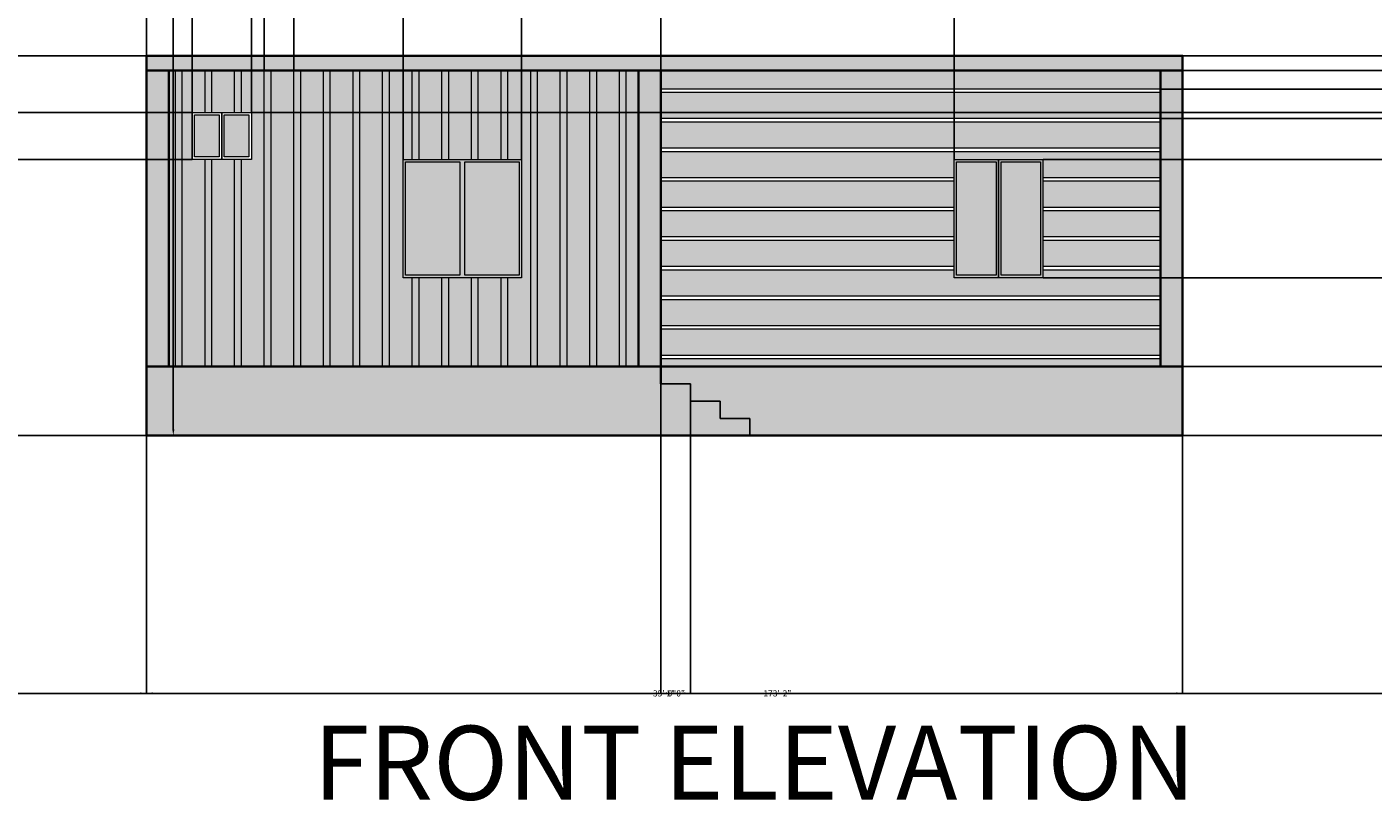
# Model space of a CAD drawing. Units: inches. Extents: x 481 to 2783, y 1975 to 3327.
# Tile 4 of 13: x 1326 to 1872, y 1975 to 2289. Entities that reach past the tile are written whole.
import ezdxf

# ---------------------------------------------------------------- set-up
doc = ezdxf.new("R2010")
doc.units = ezdxf.units.IN
doc.header["$MEASUREMENT"] = 0
for name, color, linetype, lineweight in [('A-ANNO-DIMS', 50, 'Continuous', 18), ('A-ANNO-TEXT', 50, 'Continuous', 30), ('A-ELEV', 7, 'Continuous', 35), ('A-ELEV-CLAD', 7, 'Continuous', 13), ('A-ELEV-CONC-PATT', 8, 'Continuous', 13), ('A-ELEV-FRAM-PATT', 8, 'Continuous', 13), ('A-ELEV-GLAZ', 7, 'Continuous', 20), ('A-ELEV-GLAZ-PATT', 7, 'Continuous', 13), ('A-ELEV-STRS', 7, 'Continuous', 25), ('C-TOPO', 7, 'Continuous', 25)]:
    doc.layers.add(name, color=color, linetype=linetype, lineweight=lineweight)
for name, color, linetype, lineweight, true_color in [('A-ELEV-CLAD-PATT', 141, 'Continuous', 13, 0xadddf7), ('A-ELEV-PIER-PATT', 251, 'Continuous', 13, 0x636466), ('A-ELEV-WALL-PATT', 143, 'Continuous', 13, 0x7aafdf)]:
    doc.layers.add(name, color=color, linetype=linetype, lineweight=lineweight, true_color=true_color)
doc.styles.get("Standard").update_dxf_attribs({"font": 'arial.ttf'})
doc.dimstyles.get("Standard").update_dxf_attribs({"dimtxt": 2.5, "dimasz": 2.5, "dimexe": 0.18, "dimexo": 0.0625, "dimgap": 0.09, "dimtad": 0, "dimtih": 1, "dimtoh": 1, "dimzin": 0, "dimdsep": 46, "dimlunit": 3, "dimtxsty": 'Standard', "dimcen": 0.09, "dimadec": 0, "dimazin": 0, "dimtfac": 1, "dimtofl": 0, "dimtmove": 0, "dimatfit": 3, "dimfxl": 1, "dimtolj": 1, "dimtzin": 0, "dimarcsym": 0})
pattern_1 = [(50, (0, 162.5314), (7.172602, -0.627521), [0.75, -8.25]), (355, (0, 162.531), (-1.387513, 7.521921), [0.6, -6.6]), (100.45144, (0.598, 162.479), (5.785088, 6.8944), [0.637402, -7.011421]), (46.1842, (0, 164.531), (10.672413, -1.655193), [1.125, -12.375]), (96.63564, (0.889, 164.393), (9.34662, 9.741186), [0.956103, -10.517138]), (351.18416, (0, 164.531), (9.34662, 9.741186), [0.9, -9.9]), (21, (1, 164.0314), (5.96907, -4.026189), [0.75, -8.25]), (326, (1, 164.031), (2.433153, 7.2515), [0.6, -6.6]), (71.45144, (1.4974, 163.696), (8.402224, 3.225312), [0.637402, -7.011421]), (37.5, (0, 162.5314), (0.1215986, 3.3289385), [0, -6.52, 0, -6.7, 0, -6.625]), (7.5, (0, 162.5314), (2.6306954, 3.944117), [0, -3.82, 0, -6.37, 0, -2.525]), (327.5, (-2.23, 162.5314), (5.3382244, -0.2255487), [0, -2.5, 0, -7.8, 0, -10.35]), (317.5, (-3.23, 162.5314), (5.831862, 1.00105), [0, -3.25, 0, -5.18, 0, -7.35])]

# ---------------------------------------------------------------- blocks, each defined once
blk = doc.blocks.new('*D54')
at = {"layer": 'A-ANNO-DIMS', "color": 0, "lineweight": -2, "transparency": 16777216}
for p, q in [((1324.1, 2531.22), (1385.48, 2531.22)), ((1385.3, 2528.72), (1385.3, 2328.4)), ((1385.3, 2125.32), (1385.3, 2325.64)), ((1324.1, 2122.82), (1385.48, 2122.82))]:
    blk.add_line(p, q, dxfattribs=at)
at = {"layer": 'A-ANNO-DIMS', "color": 0, "transparency": 16777216}
for points in [[(1384.88, 2528.72), (1385.72, 2528.72), (1385.3, 2531.22)], [(1384.88, 2125.32), (1385.72, 2125.32), (1385.3, 2122.82)]]:
    blk.add_solid(points, dxfattribs=at)
at = {"layer": 'Defpoints', "color": 0, "transparency": 16777216}
for p in [(1324.04, 2531.22), (1385.3, 2531.22), (1324.04, 2122.82)]:
    blk.add_point(p, dxfattribs=at)
at = {"layer": 'A-ANNO-DIMS', "color": 0, "transparency": 16777216, "insert": (1385.3, 2327.02), "char_height": 2.5, "attachment_point": 5}
blk.add_mtext('\\A1;PALM 34\'-0 1/2"', dxfattribs=at)
blk = doc.blocks.new('*D66')
at = {"layer": 'A-ANNO-DIMS', "color": 0, "lineweight": -2, "transparency": 16777216}
for p, q in [((591.06, 2122.76), (591.06, 2018.14)), ((2669.26, 2122.76), (2669.26, 2018.14)), ((593.56, 2018.32), (1624.92, 2018.32)), ((2666.76, 2018.32), (1635.4, 2018.32))]:
    blk.add_line(p, q, dxfattribs=at)
at = {"layer": 'A-ANNO-DIMS', "color": 0, "transparency": 16777216}
for points in [[(593.56, 2018.74), (593.56, 2017.9), (591.06, 2018.32)], [(2666.76, 2018.74), (2666.76, 2017.9), (2669.26, 2018.32)]]:
    blk.add_solid(points, dxfattribs=at)
at = {"layer": 'Defpoints', "color": 0, "transparency": 16777216}
for p in [(591.06, 2122.82), (2669.26, 2122.82), (2669.26, 2018.32)]:
    blk.add_point(p, dxfattribs=at)
at = {"layer": 'A-ANNO-DIMS', "color": 0, "transparency": 16777216, "insert": (1630.16, 2018.32), "char_height": 2.5, "attachment_point": 5}
blk.add_mtext('\\A1;173\'-2"', dxfattribs=at)
blk = doc.blocks.new('*D67')
at = {"layer": 'A-ANNO-DIMS', "color": 0, "lineweight": -2, "transparency": 16777216}
for p, q in [((591.06, 2122.76), (591.06, 2018.14)), ((1374.44, 2122.76), (1374.44, 2018.14)), ((593.56, 2018.32), (975.45, 2018.32)), ((1371.94, 2018.32), (990.05, 2018.32))]:
    blk.add_line(p, q, dxfattribs=at)
at = {"layer": 'A-ANNO-DIMS', "color": 0, "transparency": 16777216}
for points in [[(593.56, 2018.74), (593.56, 2017.9), (591.06, 2018.32)], [(1371.94, 2018.74), (1371.94, 2017.9), (1374.44, 2018.32)]]:
    blk.add_solid(points, dxfattribs=at)
at = {"layer": 'Defpoints', "color": 0, "transparency": 16777216}
for p in [(591.06, 2122.82), (1374.44, 2122.82), (1374.44, 2018.32)]:
    blk.add_point(p, dxfattribs=at)
at = {"layer": 'A-ANNO-DIMS', "color": 0, "transparency": 16777216, "insert": (982.75, 2018.32), "char_height": 2.5, "attachment_point": 5}
blk.add_mtext('\\A1;65\'-3 1/2"', dxfattribs=at)
blk = doc.blocks.new('*D68')
at = {"layer": 'A-ANNO-DIMS', "color": 0, "lineweight": -2, "transparency": 16777216}
for p, q in [((1374.44, 2122.76), (1374.44, 2018.14)), ((1794.44, 2122.76), (1794.44, 2018.14)), ((1376.94, 2018.32), (1580.05, 2018.32)), ((1791.94, 2018.32), (1588.82, 2018.32))]:
    blk.add_line(p, q, dxfattribs=at)
at = {"layer": 'A-ANNO-DIMS', "color": 0, "transparency": 16777216}
for points in [[(1376.94, 2018.74), (1376.94, 2017.9), (1374.44, 2018.32)], [(1791.94, 2018.74), (1791.94, 2017.9), (1794.44, 2018.32)]]:
    blk.add_solid(points, dxfattribs=at)
at = {"layer": 'Defpoints', "color": 0, "transparency": 16777216}
for p in [(1374.44, 2122.82), (1794.44, 2122.82), (1794.44, 2018.32)]:
    blk.add_point(p, dxfattribs=at)
at = {"layer": 'A-ANNO-DIMS', "color": 0, "transparency": 16777216, "insert": (1584.44, 2018.32), "char_height": 2.5, "attachment_point": 5}
blk.add_mtext('\\A1;35\'-0"', dxfattribs=at)
blk = doc.blocks.new('*D69')
at = {"layer": 'A-ANNO-DIMS', "color": 0, "lineweight": -2, "transparency": 16777216}
for p, q in [((1374.38, 2276.82), (486.38, 2276.82)), ((486.56, 2274.32), (486.56, 2201.19)), ((486.56, 2125.32), (486.56, 2198.45)), ((1374.38, 2122.82), (486.38, 2122.82))]:
    blk.add_line(p, q, dxfattribs=at)
at = {"layer": 'A-ANNO-DIMS', "color": 0, "transparency": 16777216}
for points in [[(486.15, 2274.32), (486.98, 2274.32), (486.56, 2276.82)], [(486.15, 2125.32), (486.98, 2125.32), (486.56, 2122.82)]]:
    blk.add_solid(points, dxfattribs=at)
at = {"layer": 'Defpoints', "color": 0, "transparency": 16777216}
for p in [(486.56, 2276.82), (1374.44, 2276.82), (1374.44, 2122.82)]:
    blk.add_point(p, dxfattribs=at)
at = {"layer": 'A-ANNO-DIMS', "color": 0, "transparency": 16777216, "insert": (486.56, 2199.82), "char_height": 2.5, "attachment_point": 5}
blk.add_mtext('\\A1;12\'-10"', dxfattribs=at)
blk = doc.blocks.new('*D70')
at = {"layer": 'A-ANNO-DIMS', "color": 0, "lineweight": -2, "transparency": 16777216}
for p, q in [((1794.5, 2150.82), (2773.94, 2150.82)), ((2773.76, 2148.32), (2773.76, 2138.17)), ((2773.76, 2125.32), (2773.76, 2135.48)), ((1794.5, 2122.82), (2773.94, 2122.82))]:
    blk.add_line(p, q, dxfattribs=at)
at = {"layer": 'A-ANNO-DIMS', "color": 0, "transparency": 16777216}
for points in [[(2773.34, 2148.32), (2774.17, 2148.32), (2773.76, 2150.82)], [(2773.34, 2125.32), (2774.17, 2125.32), (2773.76, 2122.82)]]:
    blk.add_solid(points, dxfattribs=at)
at = {"layer": 'Defpoints', "color": 0, "transparency": 16777216}
for p in [(1794.44, 2150.82), (2773.76, 2150.82), (1794.44, 2122.82)]:
    blk.add_point(p, dxfattribs=at)
at = {"layer": 'A-ANNO-DIMS', "color": 0, "transparency": 16777216, "insert": (2773.76, 2136.82), "char_height": 2.5, "attachment_point": 5}
blk.add_mtext('\\A1;2\'-4"', dxfattribs=at)
blk = doc.blocks.new('*D71')
at = {"layer": 'A-ANNO-DIMS', "color": 0, "lineweight": -2, "transparency": 16777216}
for p, q in [((1737.9, 2186.82), (2773.94, 2186.82)), ((2773.76, 2184.32), (2773.76, 2170.19)), ((2773.76, 2153.32), (2773.76, 2167.45)), ((1794.5, 2150.82), (2773.94, 2150.82))]:
    blk.add_line(p, q, dxfattribs=at)
at = {"layer": 'A-ANNO-DIMS', "color": 0, "transparency": 16777216}
for points in [[(2773.34, 2184.32), (2774.17, 2184.32), (2773.76, 2186.82)], [(2773.34, 2153.32), (2774.17, 2153.32), (2773.76, 2150.82)]]:
    blk.add_solid(points, dxfattribs=at)
at = {"layer": 'Defpoints', "color": 0, "transparency": 16777216}
for p in [(1737.84, 2186.82), (2773.76, 2186.82), (1794.44, 2150.82)]:
    blk.add_point(p, dxfattribs=at)
at = {"layer": 'A-ANNO-DIMS', "color": 0, "transparency": 16777216, "insert": (2773.76, 2168.82), "char_height": 2.5, "attachment_point": 5}
blk.add_mtext('\\A1;3\'-0"', dxfattribs=at)
blk = doc.blocks.new('*D72')
at = {"layer": 'A-ANNO-DIMS', "color": 0, "lineweight": -2, "transparency": 16777216}
for p, q in [((1737.9, 2234.82), (2773.94, 2234.82)), ((2773.76, 2232.32), (2773.76, 2212.19)), ((2773.76, 2189.32), (2773.76, 2209.45)), ((1737.9, 2186.82), (2773.94, 2186.82))]:
    blk.add_line(p, q, dxfattribs=at)
at = {"layer": 'A-ANNO-DIMS', "color": 0, "transparency": 16777216}
for points in [[(2773.34, 2232.32), (2774.17, 2232.32), (2773.76, 2234.82)], [(2773.34, 2189.32), (2774.17, 2189.32), (2773.76, 2186.82)]]:
    blk.add_solid(points, dxfattribs=at)
at = {"layer": 'Defpoints', "color": 0, "transparency": 16777216}
for p in [(1737.84, 2234.82), (2773.76, 2234.82), (1737.84, 2186.82)]:
    blk.add_point(p, dxfattribs=at)
at = {"layer": 'A-ANNO-DIMS', "color": 0, "transparency": 16777216, "insert": (2773.76, 2210.82), "char_height": 2.5, "attachment_point": 5}
blk.add_mtext('\\A1;4\'-0"', dxfattribs=at)
blk = doc.blocks.new('*D73')
at = {"layer": 'A-ANNO-DIMS', "color": 0, "lineweight": -2, "transparency": 16777216}
for p, q in [((1392.88, 2253.82), (486.38, 2253.82)), ((486.56, 2251.32), (486.56, 2245.67)), ((486.56, 2237.32), (486.56, 2242.98)), ((1392.88, 2234.82), (486.38, 2234.82))]:
    blk.add_line(p, q, dxfattribs=at)
at = {"layer": 'A-ANNO-DIMS', "color": 0, "transparency": 16777216}
for points in [[(486.15, 2251.32), (486.98, 2251.32), (486.56, 2253.82)], [(486.15, 2237.32), (486.98, 2237.32), (486.56, 2234.82)]]:
    blk.add_solid(points, dxfattribs=at)
at = {"layer": 'Defpoints', "color": 0, "transparency": 16777216}
for p in [(486.56, 2253.82), (1392.94, 2253.82), (1392.94, 2234.82)]:
    blk.add_point(p, dxfattribs=at)
at = {"layer": 'A-ANNO-DIMS', "color": 0, "transparency": 16777216, "insert": (486.56, 2244.32), "char_height": 2.5, "attachment_point": 5}
blk.add_mtext('\\A1;1\'-7"', dxfattribs=at)
blk = doc.blocks.new('*D74')
at = {"layer": 'A-ANNO-DIMS', "color": 0, "lineweight": -2, "transparency": 16777216}
for p, q in [((1412.86, 2270.82), (2773.94, 2270.82)), ((2773.76, 2268.32), (2773.76, 2263.69)), ((2773.76, 2256.32), (2773.76, 2260.95)), ((1417, 2253.82), (2773.94, 2253.82))]:
    blk.add_line(p, q, dxfattribs=at)
at = {"layer": 'A-ANNO-DIMS', "color": 0, "transparency": 16777216}
for points in [[(2773.34, 2268.32), (2774.17, 2268.32), (2773.76, 2270.82)], [(2773.34, 2256.32), (2774.17, 2256.32), (2773.76, 2253.82)]]:
    blk.add_solid(points, dxfattribs=at)
at = {"layer": 'Defpoints', "color": 0, "transparency": 16777216}
for p in [(1412.79, 2270.82), (2773.76, 2270.82), (1416.94, 2253.82)]:
    blk.add_point(p, dxfattribs=at)
at = {"layer": 'A-ANNO-DIMS', "color": 0, "transparency": 16777216, "insert": (2773.76, 2262.32), "char_height": 2.5, "attachment_point": 5}
blk.add_mtext('\\A1;1\'-5"', dxfattribs=at)
blk = doc.blocks.new('*D75')
at = {"layer": 'A-ANNO-DIMS', "color": 0, "lineweight": -2, "transparency": 16777216}
for p, q in [((1794.5, 2276.82), (2773.94, 2276.82)), ((2773.76, 2276.82), (2773.76, 2279.32)), ((2773.76, 2279.32), (2776.26, 2279.32)), ((1794.5, 2270.82), (2773.94, 2270.82)), ((2773.76, 2273.32), (2773.76, 2274.32))]:
    blk.add_line(p, q, dxfattribs=at)
at = {"layer": 'A-ANNO-DIMS', "color": 0, "transparency": 16777216}
for points in [[(2773.34, 2274.32), (2774.17, 2274.32), (2773.76, 2276.82)], [(2773.34, 2273.32), (2774.17, 2273.32), (2773.76, 2270.82)]]:
    blk.add_solid(points, dxfattribs=at)
at = {"layer": 'Defpoints', "color": 0, "transparency": 16777216}
for p in [(1794.44, 2276.82), (2773.76, 2276.82), (1794.44, 2270.82)]:
    blk.add_point(p, dxfattribs=at)
at = {"layer": 'A-ANNO-DIMS', "color": 0, "transparency": 16777216, "insert": (2779.67, 2279.32), "char_height": 2.5, "attachment_point": 5}
blk.add_mtext('\\A1;0\'-6"', dxfattribs=at)
blk = doc.blocks.new('*D76')
at = {"layer": 'A-ANNO-DIMS', "color": 0, "lineweight": -2, "transparency": 16777216}
for p, q in [((1374.44, 2276.88), (1374.44, 2651.23)), ((1376.94, 2651.05), (1377.48, 2651.05)), ((1390.44, 2651.05), (1389.9, 2651.05)), ((1392.94, 2253.88), (1392.94, 2651.23))]:
    blk.add_line(p, q, dxfattribs=at)
at = {"layer": 'A-ANNO-DIMS', "color": 0, "transparency": 16777216}
for points in [[(1376.94, 2651.47), (1376.94, 2650.64), (1374.44, 2651.05)], [(1390.44, 2651.47), (1390.44, 2650.64), (1392.94, 2651.05)]]:
    blk.add_solid(points, dxfattribs=at)
at = {"layer": 'Defpoints', "color": 0, "transparency": 16777216}
for p in [(1392.94, 2651.05), (1374.44, 2276.82), (1392.94, 2253.82)]:
    blk.add_point(p, dxfattribs=at)
at = {"layer": 'A-ANNO-DIMS', "color": 0, "transparency": 16777216, "insert": (1383.69, 2651.05), "char_height": 2.5, "attachment_point": 5}
blk.add_mtext('\\A1;1\'-6 1/2"', dxfattribs=at)
blk = doc.blocks.new('*D77')
at = {"layer": 'A-ANNO-DIMS', "color": 0, "lineweight": -2, "transparency": 16777216}
for p, q in [((1416.94, 2253.88), (1416.94, 2651.23)), ((1419.44, 2651.05), (1441.36, 2651.05)), ((1475.94, 2651.05), (1454.01, 2651.05)), ((1478.44, 2234.88), (1478.44, 2651.23))]:
    blk.add_line(p, q, dxfattribs=at)
at = {"layer": 'A-ANNO-DIMS', "color": 0, "transparency": 16777216}
for points in [[(1419.44, 2651.47), (1419.44, 2650.64), (1416.94, 2651.05)], [(1475.94, 2651.47), (1475.94, 2650.64), (1478.44, 2651.05)]]:
    blk.add_solid(points, dxfattribs=at)
at = {"layer": 'Defpoints', "color": 0, "transparency": 16777216}
for p in [(1478.44, 2651.05), (1416.94, 2253.82), (1478.44, 2234.82)]:
    blk.add_point(p, dxfattribs=at)
at = {"layer": 'A-ANNO-DIMS', "color": 0, "transparency": 16777216, "insert": (1447.69, 2651.05), "char_height": 2.5, "attachment_point": 5}
blk.add_mtext('\\A1;5\'-1 1/2"', dxfattribs=at)
blk = doc.blocks.new('*D78')
at = {"layer": 'A-ANNO-DIMS', "color": 0, "lineweight": -2, "transparency": 16777216}
for p, q in [((1526.44, 2234.88), (1526.44, 2651.23)), ((1528.94, 2651.05), (1548.31, 2651.05)), ((1580.44, 2651.05), (1561.06, 2651.05)), ((1582.94, 2270.88), (1582.94, 2651.23))]:
    blk.add_line(p, q, dxfattribs=at)
at = {"layer": 'A-ANNO-DIMS', "color": 0, "transparency": 16777216}
for points in [[(1528.94, 2651.47), (1528.94, 2650.64), (1526.44, 2651.05)], [(1580.44, 2651.47), (1580.44, 2650.64), (1582.94, 2651.05)]]:
    blk.add_solid(points, dxfattribs=at)
at = {"layer": 'Defpoints', "color": 0, "transparency": 16777216}
for p in [(1582.94, 2651.05), (1582.94, 2270.82), (1526.44, 2234.82)]:
    blk.add_point(p, dxfattribs=at)
at = {"layer": 'A-ANNO-DIMS', "color": 0, "transparency": 16777216, "insert": (1554.69, 2651.05), "char_height": 2.5, "attachment_point": 5}
blk.add_mtext('\\A1;4\'-8 1/2"', dxfattribs=at)
blk = doc.blocks.new('*D79')
at = {"layer": 'A-ANNO-DIMS', "color": 0, "lineweight": -2, "transparency": 16777216}
for p, q in [((1582.94, 2270.88), (1582.94, 2651.23)), ((1585.44, 2651.05), (1638.01, 2651.05)), ((1699.34, 2651.05), (1646.77, 2651.05)), ((1701.84, 2234.88), (1701.84, 2651.23))]:
    blk.add_line(p, q, dxfattribs=at)
at = {"layer": 'A-ANNO-DIMS', "color": 0, "transparency": 16777216}
for points in [[(1585.44, 2651.47), (1585.44, 2650.64), (1582.94, 2651.05)], [(1699.34, 2651.47), (1699.34, 2650.64), (1701.84, 2651.05)]]:
    blk.add_solid(points, dxfattribs=at)
at = {"layer": 'Defpoints', "color": 0, "transparency": 16777216}
for p in [(1701.84, 2651.05), (1582.94, 2270.82), (1701.84, 2234.82)]:
    blk.add_point(p, dxfattribs=at)
at = {"layer": 'A-ANNO-DIMS', "color": 0, "transparency": 16777216, "insert": (1642.39, 2651.05), "char_height": 2.5, "attachment_point": 5}
blk.add_mtext('\\A1;9\'-11"', dxfattribs=at)
blk = doc.blocks.new('*D80')
at = {"layer": 'A-ANNO-DIMS', "color": 0, "lineweight": -2, "transparency": 16777216}
for p, q in [((1582.94, 2150.76), (1582.94, 2018.14)), ((1594.94, 2143.76), (1594.94, 2018.14)), ((1585.44, 2018.32), (1585.64, 2018.32)), ((1592.44, 2018.32), (1592.23, 2018.32))]:
    blk.add_line(p, q, dxfattribs=at)
at = {"layer": 'A-ANNO-DIMS', "color": 0, "transparency": 16777216}
for points in [[(1585.44, 2018.74), (1585.44, 2017.9), (1582.94, 2018.32)], [(1592.44, 2018.74), (1592.44, 2017.9), (1594.94, 2018.32)]]:
    blk.add_solid(points, dxfattribs=at)
at = {"layer": 'Defpoints', "color": 0, "transparency": 16777216}
for p in [(1582.94, 2150.82), (1594.94, 2143.82), (1582.94, 2018.32)]:
    blk.add_point(p, dxfattribs=at)
at = {"layer": 'A-ANNO-DIMS', "color": 0, "transparency": 16777216, "insert": (1588.94, 2018.32), "char_height": 2.5, "attachment_point": 5}
blk.add_mtext('\\A1;1\'-0"', dxfattribs=at)
blk = doc.blocks.new('*D81')
at = {"layer": 'A-ANNO-DIMS', "color": 0, "lineweight": -2, "transparency": 16777216}
for p, q in [((1422.16, 2270.88), (1422.16, 2651.23)), ((1424.66, 2651.05), (1424.87, 2651.05)), ((1431.66, 2651.05), (1431.46, 2651.05)), ((1434.16, 2270.88), (1434.16, 2651.23))]:
    blk.add_line(p, q, dxfattribs=at)
at = {"layer": 'A-ANNO-DIMS', "color": 0, "transparency": 16777216}
for points in [[(1424.66, 2651.47), (1424.66, 2650.64), (1422.16, 2651.05)], [(1431.66, 2651.47), (1431.66, 2650.64), (1434.16, 2651.05)]]:
    blk.add_solid(points, dxfattribs=at)
at = {"layer": 'Defpoints', "color": 0, "transparency": 16777216}
for p in [(1434.16, 2651.05), (1422.16, 2270.82), (1434.16, 2270.82)]:
    blk.add_point(p, dxfattribs=at)
at = {"layer": 'A-ANNO-DIMS', "color": 0, "transparency": 16777216, "insert": (1428.16, 2651.05), "char_height": 2.5, "attachment_point": 5}
blk.add_mtext('\\A1;1\'-0"', dxfattribs=at)
blk = doc.blocks.new('*D82')
at = {"layer": 'A-ANNO-DIMS', "color": 0, "lineweight": -2, "transparency": 16777216}
for p, q in [((1785.5, 2263.36), (2773.94, 2263.36)), ((2773.76, 2260.86), (2773.76, 2258.72)), ((2773.76, 2253.86), (2773.76, 2255.99)), ((1785.5, 2251.36), (2773.94, 2251.36))]:
    blk.add_line(p, q, dxfattribs=at)
at = {"layer": 'A-ANNO-DIMS', "color": 0, "transparency": 16777216}
for points in [[(2773.34, 2260.86), (2774.17, 2260.86), (2773.76, 2263.36)], [(2773.34, 2253.86), (2774.17, 2253.86), (2773.76, 2251.36)]]:
    blk.add_solid(points, dxfattribs=at)
at = {"layer": 'Defpoints', "color": 0, "transparency": 16777216}
for p in [(1785.44, 2263.36), (1785.44, 2251.36), (2773.76, 2251.36)]:
    blk.add_point(p, dxfattribs=at)
at = {"layer": 'A-ANNO-DIMS', "color": 0, "transparency": 16777216, "insert": (2773.76, 2257.36), "char_height": 2.5, "attachment_point": 5}
blk.add_mtext('\\A1;1\'-0"', dxfattribs=at)

msp = doc.modelspace()

# ---------------------------------------------------------------- hatches: boundary and pattern name
at = {"layer": 'A-ELEV-CLAD-PATT'}
h = msp.add_hatch(color=256, dxfattribs=at)
h.paths.add_polyline_path([(1386.162, 2150.821), (1388.793, 2150.821), (1388.793, 2270.821), (1386.162, 2270.821)])
h.paths.add_polyline_path([(1398.162, 2150.821), (1400.793, 2150.821), (1400.793, 2234.821), (1398.162, 2234.821)])
h.paths.add_polyline_path([(1410.162, 2150.821), (1412.793, 2150.821), (1412.793, 2234.821), (1410.162, 2234.821)])
h.paths.add_polyline_path([(1422.162, 2150.821), (1424.793, 2150.821), (1424.793, 2270.821), (1422.162, 2270.821)])
h.paths.add_polyline_path([(1436.793, 2270.821), (1434.162, 2270.821), (1434.162, 2150.821), (1436.793, 2150.821)])
h.paths.add_polyline_path([(1446.162, 2150.821), (1448.793, 2150.821), (1448.793, 2270.821), (1446.162, 2270.821)])
h.paths.add_polyline_path([(1460.793, 2270.821), (1458.162, 2270.821), (1458.162, 2150.821), (1460.793, 2150.821)])
h.paths.add_polyline_path([(1470.162, 2150.821), (1472.793, 2150.821), (1472.793, 2270.821), (1470.162, 2270.821)])
h.paths.add_polyline_path([(1484.793, 2270.821), (1482.162, 2270.821), (1482.162, 2234.821), (1484.793, 2234.821)])
h.paths.add_polyline_path([(1494.162, 2234.821), (1496.793, 2234.821), (1496.793, 2270.821), (1494.162, 2270.821)])
h.paths.add_polyline_path([(1508.793, 2270.821), (1506.162, 2270.821), (1506.162, 2234.821), (1508.793, 2234.821)])
h.paths.add_polyline_path([(1520.793, 2270.821), (1518.162, 2270.821), (1518.162, 2234.821), (1520.793, 2234.821)])
h.paths.add_polyline_path([(1532.793, 2270.821), (1530.162, 2270.821), (1530.162, 2150.821), (1532.793, 2150.821)])
h.paths.add_polyline_path([(1544.793, 2270.821), (1542.162, 2270.821), (1542.162, 2150.821), (1544.793, 2150.821)])
h.paths.add_polyline_path([(1556.793, 2270.821), (1554.162, 2270.821), (1554.162, 2150.821), (1556.793, 2150.821)])
h.paths.add_polyline_path([(1568.793, 2270.821), (1566.162, 2270.821), (1566.162, 2150.821), (1568.793, 2150.821)])
h.paths.add_polyline_path([(1484.793, 2186.821), (1482.162, 2186.821), (1482.162, 2150.821), (1484.793, 2150.821)])
h.paths.add_polyline_path([(1496.793, 2186.821), (1494.162, 2186.821), (1494.162, 2150.821), (1496.793, 2150.821)])
h.paths.add_polyline_path([(1508.793, 2186.821), (1506.162, 2186.821), (1506.162, 2150.821), (1508.793, 2150.821)])
h.paths.add_polyline_path([(1520.793, 2186.821), (1518.162, 2186.821), (1518.162, 2150.821), (1520.793, 2150.821)])
h.paths.add_polyline_path([(1398.162, 2253.821), (1400.793, 2253.821), (1400.793, 2270.821), (1398.162, 2270.821)])
h.paths.add_polyline_path([(1410.162, 2253.821), (1412.793, 2253.821), (1412.793, 2270.821), (1410.162, 2270.821)])
at = {"layer": 'A-ELEV-CONC-PATT'}
h = msp.add_hatch(dxfattribs=at)
h.set_pattern_fill('AR-CONC', color=256, style=0)
h.set_pattern_definition(pattern_1)
h.paths.add_polyline_path([(1794.438, 2270.821), (1794.438, 2276.821), (1374.438, 2276.821), (1374.438, 2270.821)])
h = msp.add_hatch(dxfattribs=at)
h.set_pattern_fill('AR-CONC', color=256, style=0)
h.set_pattern_definition(pattern_1)
h.paths.add_polyline_path([(1594.938, 2143.821), (1582.938, 2143.821), (1582.938, 2150.821), (1570.938, 2150.821), (1374.438, 2150.821), (1374.438, 2122.821), (1618.938, 2122.821), (1618.938, 2129.821), (1606.938, 2129.821), (1606.938, 2136.821), (1594.938, 2136.821)])
h.paths.add_polyline_path([(1794.438, 2150.821), (1582.938, 2150.821), (1582.938, 2143.821), (1594.938, 2143.821), (1594.938, 2136.821), (1606.938, 2136.821), (1606.938, 2129.821), (1618.938, 2129.821), (1618.938, 2122.821), (1794.438, 2122.821)])
at = {"layer": 'A-ELEV-FRAM-PATT'}
h = msp.add_hatch(color=256, dxfattribs=at)
h.paths.add_polyline_path([(1526.438, 2234.821), (1502.438, 2234.821), (1478.438, 2234.821), (1478.438, 2186.821), (1502.438, 2186.821), (1526.438, 2186.821)])
h.paths.add_polyline_path([(1501.438, 2233.821), (1501.438, 2187.821), (1479.438, 2187.821), (1479.438, 2233.821)], flags=16)
h.paths.add_polyline_path([(1503.438, 2233.821), (1525.438, 2233.821), (1525.438, 2187.821), (1503.438, 2187.821)], flags=16)
h.paths.add_polyline_path([(1719.842, 2234.821), (1701.842, 2234.821), (1701.842, 2186.821), (1719.842, 2186.821)])
h.paths.add_polyline_path([(1718.842, 2233.821), (1718.842, 2187.821), (1702.842, 2187.821), (1702.842, 2233.821)], flags=16)
h.paths.add_polyline_path([(1737.842, 2234.821), (1719.842, 2234.821), (1719.842, 2186.821), (1737.842, 2186.821)])
h.paths.add_polyline_path([(1736.842, 2233.821), (1736.842, 2187.821), (1720.842, 2187.821), (1720.842, 2233.821)], flags=16)
at = {"layer": 'A-ELEV-GLAZ-PATT'}
h = msp.add_hatch(color=256, dxfattribs=at)
h.set_gradient(color1=(254, 204, 102), color2=(255, 255, 0), tint=1)
h.paths.add_polyline_path([(1479.438, 2187.821), (1501.438, 2187.821), (1501.438, 2233.821), (1479.438, 2233.821)])
h.paths.add_polyline_path([(1503.438, 2187.821), (1525.438, 2187.821), (1525.438, 2233.821), (1503.438, 2233.821)])
h.paths.add_polyline_path([(1702.842, 2187.821), (1718.842, 2187.821), (1718.842, 2233.821), (1702.842, 2233.821)])
h.paths.add_polyline_path([(1720.842, 2187.821), (1736.842, 2187.821), (1736.842, 2233.821), (1720.842, 2233.821)])
at = {"layer": 'A-ELEV-PIER-PATT'}
h = msp.add_hatch(color=256, dxfattribs=at)
h.paths.add_polyline_path([(1374.438, 2150.821), (1383.438, 2150.821), (1383.438, 2270.821), (1374.438, 2270.821)])
h.paths.add_polyline_path([(1582.938, 2270.821), (1573.938, 2270.821), (1573.938, 2150.821), (1582.938, 2150.821)])
h.paths.add_polyline_path([(1794.438, 2270.821), (1785.438, 2270.821), (1785.438, 2150.821), (1794.438, 2150.821)])
at = {"layer": 'A-ELEV-WALL-PATT'}
msp.add_hatch(color=256, dxfattribs=at).paths.add_polyline_path([(1383.438, 2150.821), (1386.162, 2150.821), (1386.162, 2270.821), (1383.438, 2270.821)])
h = msp.add_hatch(color=256, dxfattribs=at)
h.paths.add_polyline_path([(1398.162, 2234.821), (1392.938, 2234.821), (1392.938, 2253.821), (1398.162, 2253.821), (1398.162, 2270.821), (1388.793, 2270.821), (1388.793, 2150.821), (1398.162, 2150.821)])
h.paths.add_polyline_path([(1400.793, 2150.821), (1410.162, 2150.821), (1410.162, 2234.821), (1404.938, 2234.821), (1400.793, 2234.821)])
h.paths.add_polyline_path([(1400.793, 2253.821), (1404.938, 2253.821), (1410.162, 2253.821), (1410.162, 2270.821), (1400.793, 2270.821)])
h.paths.add_polyline_path([(1412.793, 2253.821), (1416.938, 2253.821), (1416.938, 2234.821), (1412.793, 2234.821), (1412.793, 2150.821), (1422.162, 2150.821), (1422.162, 2270.821), (1412.793, 2270.821)])
h.paths.add_polyline_path([(1424.793, 2150.821), (1434.162, 2150.821), (1434.162, 2210.821), (1434.162, 2270.821), (1424.793, 2270.821)])
h.paths.add_polyline_path([(1436.793, 2150.821), (1446.162, 2150.821), (1446.162, 2210.821), (1446.162, 2270.821), (1436.793, 2270.821)])
h.paths.add_polyline_path([(1448.793, 2150.821), (1458.162, 2150.821), (1458.162, 2210.821), (1458.162, 2270.821), (1448.793, 2270.821)])
h.paths.add_polyline_path([(1470.162, 2270.821), (1460.793, 2270.821), (1460.793, 2150.821), (1470.162, 2150.821), (1470.162, 2204.821)])
h.paths.add_polyline_path([(1482.162, 2270.821), (1472.793, 2270.821), (1472.793, 2150.821), (1482.162, 2150.821), (1482.162, 2186.821), (1478.438, 2186.821), (1478.438, 2234.821), (1482.162, 2234.821)])
h.paths.add_polyline_path([(1484.793, 2234.821), (1494.162, 2234.821), (1494.162, 2270.821), (1484.793, 2270.821)])
h.paths.add_polyline_path([(1506.162, 2270.821), (1496.793, 2270.821), (1496.793, 2234.821), (1502.438, 2234.821), (1506.162, 2234.821)])
h.paths.add_polyline_path([(1508.793, 2234.821), (1518.162, 2234.821), (1518.162, 2270.821), (1508.793, 2270.821)])
h.paths.add_polyline_path([(1520.793, 2234.821), (1526.438, 2234.821), (1526.438, 2186.821), (1520.793, 2186.821), (1520.793, 2150.821), (1530.162, 2150.821), (1530.162, 2270.821), (1520.793, 2270.821)])
h.paths.add_polyline_path([(1542.162, 2270.821), (1532.793, 2270.821), (1532.793, 2150.821), (1542.162, 2150.821)])
h.paths.add_polyline_path([(1554.162, 2270.821), (1544.793, 2270.821), (1544.793, 2150.821), (1554.162, 2150.821)])
h.paths.add_polyline_path([(1556.793, 2150.821), (1566.162, 2150.821), (1566.162, 2270.821), (1558.938, 2270.821), (1556.793, 2270.821)])
h.paths.add_polyline_path([(1568.793, 2150.821), (1573.938, 2150.821), (1573.938, 2270.821), (1568.793, 2270.821)])
h.paths.add_polyline_path([(1484.793, 2150.821), (1494.162, 2150.821), (1494.162, 2186.821), (1484.793, 2186.821)])
h.paths.add_polyline_path([(1506.162, 2186.821), (1502.438, 2186.821), (1498.938, 2186.821), (1496.793, 2186.821), (1496.793, 2150.821), (1506.162, 2150.821)])
h.paths.add_polyline_path([(1508.793, 2150.821), (1518.162, 2150.821), (1518.162, 2186.821), (1508.793, 2186.821)])
h = msp.add_hatch(color=256, dxfattribs=at)
h.set_gradient(color1=(237, 31, 36), color2=(242, 113, 114), tint=1)
h.paths.add_polyline_path([(1393.938, 2235.821), (1403.938, 2235.821), (1403.938, 2252.821), (1393.938, 2252.821)])
h.paths.add_polyline_path([(1405.938, 2235.821), (1415.938, 2235.821), (1415.938, 2252.821), (1405.938, 2252.821)])
h.paths.add_polyline_path([(1785.438, 2263.356), (1785.438, 2270.821), (1582.938, 2270.821), (1582.938, 2263.356)])
h.paths.add_polyline_path([(1785.438, 2251.356), (1785.438, 2262.06), (1582.938, 2262.06), (1582.938, 2251.356)])
h.paths.add_polyline_path([(1785.438, 2239.356), (1785.438, 2250.06), (1582.938, 2250.06), (1582.938, 2239.356)])
h.paths.add_polyline_path([(1701.842, 2227.356), (1701.842, 2234.821), (1719.842, 2234.821), (1737.842, 2234.821), (1737.842, 2227.356), (1785.438, 2227.356), (1785.438, 2238.06), (1582.938, 2238.06), (1582.938, 2227.356)])
h.paths.add_polyline_path([(1701.842, 2215.356), (1701.842, 2226.06), (1582.938, 2226.06), (1582.938, 2215.356)])
h.paths.add_polyline_path([(1701.842, 2203.356), (1701.842, 2214.06), (1582.938, 2214.06), (1582.938, 2203.356)])
h.paths.add_polyline_path([(1701.842, 2191.356), (1701.842, 2202.06), (1582.938, 2202.06), (1582.938, 2191.356)])
h.paths.add_polyline_path([(1785.438, 2179.356), (1785.438, 2190.06), (1737.842, 2190.06), (1737.842, 2186.821), (1719.842, 2186.821), (1701.842, 2186.821), (1701.842, 2190.06), (1582.938, 2190.06), (1582.938, 2179.356)])
h.paths.add_polyline_path([(1785.438, 2167.356), (1785.438, 2178.06), (1582.938, 2178.06), (1582.938, 2167.356)])
h.paths.add_polyline_path([(1785.438, 2155.356), (1785.438, 2166.06), (1582.938, 2166.06), (1582.938, 2155.356)])
h.paths.add_polyline_path([(1737.842, 2202.06), (1737.842, 2191.356), (1785.438, 2191.356), (1785.438, 2202.06)])
h.paths.add_polyline_path([(1737.842, 2214.06), (1737.842, 2203.356), (1785.438, 2203.356), (1785.438, 2214.06)])
h.paths.add_polyline_path([(1785.438, 2215.356), (1785.438, 2226.06), (1737.842, 2226.06), (1737.842, 2215.356)])
h.paths.add_polyline_path([(1582.938, 2154.06), (1582.938, 2150.821), (1785.438, 2150.821), (1785.438, 2154.06)])

# ---------------------------------------------------------------- linework, layer by layer
at = {"layer": 'A-ELEV'}
for p, q in [((1374.438, 2276.821), (1374.438, 2122.821)), ((1794.438, 2276.821), (1374.438, 2276.821)), ((1374.438, 2276.821), (1374.438, 2270.821)), ((1570.938, 2276.821), (1582.938, 2276.821)), ((1794.438, 2276.821), (1794.438, 2122.821)), ((1794.438, 2276.821), (1794.438, 2270.821)), ((1794.438, 2270.821), (1374.438, 2270.821)), ((1383.438, 2270.821), (1383.438, 2150.821)), ((1558.938, 2270.821), (1570.938, 2270.821)), ((1573.938, 2150.821), (1573.938, 2270.821)), ((1582.938, 2143.821), (1582.938, 2270.821)), ((1785.438, 2270.821), (1785.438, 2150.821)), ((1794.438, 2150.821), (1374.438, 2150.821)), ((1794.438, 2122.821), (1374.438, 2122.821))]:
    msp.add_line(p, q, dxfattribs=at)
msp.add_lwpolyline([(1374.438, 2276.821), (1794.438, 2276.821), (1794.438, 2276.821), (1374.438, 2276.821)], close=True, dxfattribs=at)
at = {"layer": 'A-ELEV-CLAD'}
for p, q in [((1383.438, 2270.821), (1386.162, 2270.821)), ((1383.438, 2150.821), (1386.162, 2150.821))]:
    msp.add_line(p, q, dxfattribs=at)
for points in [[(1386.162, 2270.821), (1388.793, 2270.821), (1388.793, 2150.821), (1386.162, 2150.821)], [(1422.162, 2270.821), (1424.793, 2270.821), (1424.793, 2150.821), (1422.162, 2150.821)], [(1530.162, 2270.821), (1532.793, 2270.821), (1532.793, 2150.821), (1530.162, 2150.821)], [(1542.162, 2270.821), (1544.793, 2270.821), (1544.793, 2150.821), (1542.162, 2150.821)], [(1554.162, 2270.821), (1556.793, 2270.821), (1556.793, 2150.821), (1554.162, 2150.821)], [(1566.162, 2270.821), (1568.793, 2270.821), (1568.793, 2150.821), (1566.162, 2150.821)], [(1582.938, 2262.06), (1785.438, 2262.06), (1785.438, 2263.356), (1582.938, 2263.356)], [(1582.938, 2250.06), (1785.438, 2250.06), (1785.438, 2251.356), (1582.938, 2251.356)], [(1582.938, 2238.06), (1785.438, 2238.06), (1785.438, 2239.356), (1582.938, 2239.356)], [(1582.938, 2178.06), (1785.438, 2178.06), (1785.438, 2179.356), (1582.938, 2179.356)], [(1582.938, 2166.06), (1785.438, 2166.06), (1785.438, 2167.356), (1582.938, 2167.356)], [(1582.938, 2154.06), (1785.438, 2154.06), (1785.438, 2155.356), (1582.938, 2155.356)]]:
    msp.add_lwpolyline(points, close=True, dxfattribs=at)
for points in [[(1398.162, 2253.821), (1398.162, 2270.821), (1400.793, 2270.821), (1400.793, 2253.821)], [(1410.162, 2253.821), (1410.162, 2270.821), (1412.793, 2270.821), (1412.793, 2253.821)], [(1434.162, 2150.821), (1434.162, 2270.821), (1436.793, 2270.821), (1436.793, 2150.821)], [(1446.162, 2150.821), (1446.162, 2270.821), (1448.793, 2270.821), (1448.793, 2150.821)], [(1458.162, 2150.821), (1458.162, 2270.821), (1460.793, 2270.821), (1460.793, 2150.821)], [(1470.162, 2150.821), (1470.162, 2270.821), (1472.793, 2270.821), (1472.793, 2150.821)], [(1482.162, 2234.821), (1482.162, 2270.821), (1484.793, 2270.821), (1484.793, 2234.821)], [(1494.162, 2234.821), (1494.162, 2270.821), (1496.793, 2270.821), (1496.793, 2234.821)], [(1506.162, 2234.821), (1506.162, 2270.821), (1508.793, 2270.821), (1508.793, 2234.821)], [(1518.162, 2234.821), (1518.162, 2270.821), (1520.793, 2270.821), (1520.793, 2234.821)], [(1400.793, 2234.821), (1400.793, 2150.821), (1398.162, 2150.821), (1398.162, 2234.821)], [(1412.793, 2234.821), (1412.793, 2150.821), (1410.162, 2150.821), (1410.162, 2234.821)], [(1701.842, 2227.356), (1582.938, 2227.356), (1582.938, 2226.06), (1701.842, 2226.06)], [(1737.842, 2226.06), (1785.438, 2226.06), (1785.438, 2227.356), (1737.842, 2227.356)], [(1436.793, 2210.821), (1436.793, 2150.821), (1434.162, 2150.821), (1434.162, 2210.821)], [(1448.793, 2210.821), (1448.793, 2150.821), (1446.162, 2150.821), (1446.162, 2210.821)], [(1460.793, 2210.821), (1460.793, 2150.821), (1458.162, 2150.821), (1458.162, 2210.821)], [(1701.842, 2215.356), (1582.938, 2215.356), (1582.938, 2214.06), (1701.842, 2214.06)], [(1737.842, 2214.06), (1785.438, 2214.06), (1785.438, 2215.356), (1737.842, 2215.356)], [(1472.793, 2204.821), (1472.793, 2150.821), (1470.162, 2150.821), (1470.162, 2204.821)], [(1701.842, 2203.356), (1582.938, 2203.356), (1582.938, 2202.06), (1701.842, 2202.06)], [(1737.842, 2202.06), (1785.438, 2202.06), (1785.438, 2203.356), (1737.842, 2203.356)], [(1701.842, 2191.356), (1582.938, 2191.356), (1582.938, 2190.06), (1701.842, 2190.06)], [(1737.842, 2190.06), (1785.438, 2190.06), (1785.438, 2191.356), (1737.842, 2191.356)], [(1484.793, 2186.821), (1484.793, 2150.821), (1482.162, 2150.821), (1482.162, 2186.821)], [(1496.793, 2186.821), (1496.793, 2150.821), (1494.162, 2150.821), (1494.162, 2186.821)], [(1508.793, 2186.821), (1508.793, 2150.821), (1506.162, 2150.821), (1506.162, 2186.821)], [(1520.793, 2186.821), (1520.793, 2150.821), (1518.162, 2150.821), (1518.162, 2186.821)]]:
    msp.add_lwpolyline(points, dxfattribs=at)
at = {"layer": 'A-ELEV-GLAZ'}
for p, q in [((1392.938, 2253.821), (1392.938, 2234.821)), ((1486.938, 2234.821), (1498.938, 2234.821)), ((1510.938, 2186.821), (1498.938, 2186.821))]:
    msp.add_line(p, q, dxfattribs=at)
for points in [[(1392.938, 2253.821), (1416.938, 2253.821), (1416.938, 2234.821), (1392.938, 2234.821)], [(1502.438, 2186.821), (1478.438, 2186.821), (1478.438, 2234.821), (1502.438, 2234.821)], [(1502.438, 2234.821), (1526.438, 2234.821), (1526.438, 2186.821), (1502.438, 2186.821)]]:
    msp.add_lwpolyline(points, dxfattribs=at)
for points in [[(1392.938, 2253.821), (1404.938, 2253.821), (1404.938, 2234.821), (1392.938, 2234.821)], [(1404.938, 2253.821), (1416.938, 2253.821), (1416.938, 2234.821), (1404.938, 2234.821)], [(1393.938, 2252.821), (1403.938, 2252.821), (1403.938, 2235.821), (1393.938, 2235.821)], [(1405.938, 2252.821), (1415.938, 2252.821), (1415.938, 2235.821), (1405.938, 2235.821)], [(1478.438, 2234.821), (1526.438, 2234.821), (1526.438, 2186.821), (1478.438, 2186.821)], [(1479.438, 2233.821), (1501.438, 2233.821), (1501.438, 2187.821), (1479.438, 2187.821)], [(1503.438, 2233.821), (1525.438, 2233.821), (1525.438, 2187.821), (1503.438, 2187.821)], [(1701.842, 2234.821), (1737.842, 2234.821), (1737.842, 2186.821), (1701.842, 2186.821)], [(1701.842, 2234.821), (1719.842, 2234.821), (1719.842, 2186.821), (1701.842, 2186.821)], [(1702.842, 2233.821), (1718.842, 2233.821), (1718.842, 2187.821), (1702.842, 2187.821)], [(1719.842, 2234.821), (1737.842, 2234.821), (1737.842, 2186.821), (1719.842, 2186.821)], [(1720.842, 2233.821), (1736.842, 2233.821), (1736.842, 2187.821), (1720.842, 2187.821)]]:
    msp.add_lwpolyline(points, close=True, dxfattribs=at)
at = {"layer": 'A-ELEV-STRS'}
for p, q in [((1582.938, 2150.821), (1570.938, 2150.821)), ((1582.938, 2143.821), (1582.938, 2150.821)), ((1594.938, 2143.821), (1582.938, 2143.821)), ((1594.938, 2136.821), (1594.938, 2143.821)), ((1606.938, 2136.821), (1594.938, 2136.821)), ((1606.938, 2129.821), (1606.938, 2136.821)), ((1618.938, 2129.821), (1606.938, 2129.821)), ((1618.938, 2122.821), (1618.938, 2129.821))]:
    msp.add_line(p, q, dxfattribs=at)
at = {"layer": 'C-TOPO'}
for p, q in [((1374.438, 2122.821), (591.063, 2122.821)), ((1794.438, 2122.821), (2669.257, 2122.821))]:
    msp.add_line(p, q, dxfattribs=at)

# ---------------------------------------------------------------- texts
at = {"layer": 'A-ANNO-TEXT', "insert": (1442.085, 2005.182), "char_height": 30, "attachment_point": 1}
msp.add_mtext_dynamic_manual_height_columns('FRONT ELEVATION', width=395.6916, gutter_width=1, heights=[0], dxfattribs=at)

# ---------------------------------------------------------------- dimensions: what is measured, and where the dimension line sits
at = {"layer": 'A-ANNO-DIMS'}
for base, p1, p2, picture, middle in [((1392.938, 2651.053), (1374.438, 2276.821), (1392.938, 2253.821), '*D76', (1383.688, 2651.053)), ((1478.438, 2651.053), (1416.938, 2253.821), (1478.438, 2234.821), '*D77', (1447.688, 2651.053)), ((1434.162, 2651.053), (1422.162, 2270.821), (1434.162, 2270.821), '*D81', (1428.162, 2651.053)), ((1582.938, 2651.053), (1526.438, 2234.821), (1582.938, 2270.821), '*D78', (1554.688, 2651.053)), ((1701.842, 2651.053), (1582.938, 2270.821), (1701.842, 2234.821), '*D79', (1642.39, 2651.053)), ((1582.938, 2018.321), (1594.938, 2143.821), (1582.938, 2150.821), '*D80', (1588.938, 2018.321)), ((2669.257, 2018.321), (591.063, 2122.821), (2669.257, 2122.821), '*D66', (1630.16, 2018.321)), ((1374.438, 2018.321), (591.063, 2122.821), (1374.438, 2122.821), '*D67', (982.75, 2018.321)), ((1794.438, 2018.321), (1374.438, 2122.821), (1794.438, 2122.821), '*D68', (1584.438, 2018.321))]:
    dim = msp.add_linear_dim(base=base, p1=p1, p2=p2, dimstyle='Standard', override={"dimdec": 1, "dimlfac": 1, "dimrnd": 0, "dimzin": 1, "dimdsep": 46, "dimlunit": 4, "dimfrac": 2}, dxfattribs=at)
    dim.commit()
    dim.dimension.update_dxf_attribs({"geometry": picture, "text_midpoint": middle})
dim = msp.add_linear_dim(base=(1385.301, 2531.217), p1=(1324.042, 2122.821), p2=(1324.042, 2531.217), angle=90, text='PALM <>', dimstyle='Standard', override={"dimdec": 1, "dimlfac": 1, "dimrnd": 0, "dimzin": 1, "dimdsep": 46, "dimlunit": 4, "dimfrac": 2}, dxfattribs=at)
dim.commit()
dim.dimension.update_dxf_attribs({"geometry": '*D54', "text_midpoint": (1385.301, 2327.019)})
for base, p1, p2, picture, middle in [((2773.757, 2276.821), (1794.438, 2270.821), (1794.438, 2276.821), '*D75', (2779.67, 2279.321)), ((486.563, 2276.821), (1374.438, 2122.821), (1374.438, 2276.821), '*D69', (486.563, 2199.821)), ((2773.757, 2270.821), (1416.938, 2253.821), (1412.793, 2270.821), '*D74', (2773.757, 2262.321)), ((2773.757, 2251.356), (1785.438, 2263.356), (1785.438, 2251.356), '*D82', (2773.757, 2257.356)), ((486.563, 2253.821), (1392.938, 2234.821), (1392.938, 2253.821), '*D73', (486.563, 2244.321)), ((2773.757, 2234.821), (1737.842, 2186.821), (1737.842, 2234.821), '*D72', (2773.757, 2210.821)), ((2773.757, 2186.821), (1794.438, 2150.821), (1737.842, 2186.821), '*D71', (2773.757, 2168.821)), ((2773.757, 2150.821), (1794.438, 2122.821), (1794.438, 2150.821), '*D70', (2773.757, 2136.821))]:
    dim = msp.add_linear_dim(base=base, p1=p1, p2=p2, angle=90, dimstyle='Standard', override={"dimdec": 1, "dimlfac": 1, "dimrnd": 0, "dimzin": 1, "dimdsep": 46, "dimlunit": 4, "dimfrac": 2}, dxfattribs=at)
    dim.commit()
    dim.dimension.update_dxf_attribs({"geometry": picture, "text_midpoint": middle})

doc.saveas('drawing.dxf')
